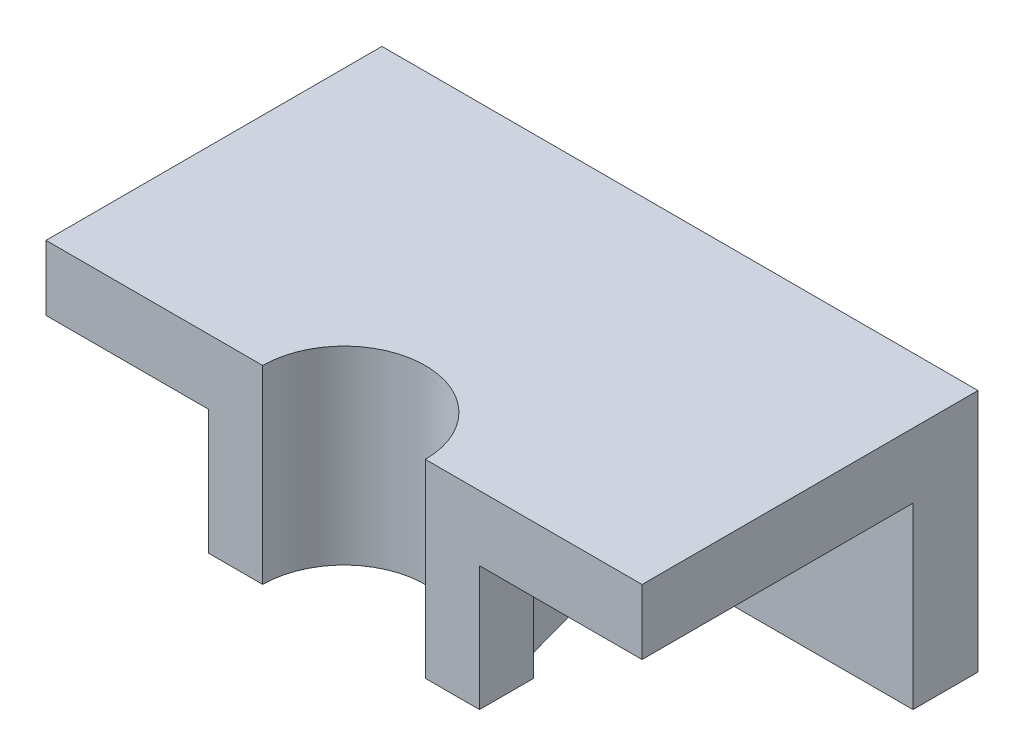
ISO-10303-21;
HEADER;
FILE_DESCRIPTION(('STEP AP214'),'2;1');
FILE_NAME('part.step','',(''),(''),'','','');
FILE_SCHEMA(('AUTOMOTIVE_DESIGN { 1 0 10303 214 1 1 1 1 }'));
ENDSEC;
DATA;
#1=APPLICATION_CONTEXT('core data for automotive mechanical design processes');
#2=APPLICATION_PROTOCOL_DEFINITION('international standard','automotive_design',2000,#1);
#3=PRODUCT_CONTEXT('',#1,'mechanical');
#4=PRODUCT('Part','Part','',(#3));
#5=PRODUCT_RELATED_PRODUCT_CATEGORY('part','',(#4));
#6=PRODUCT_DEFINITION_FORMATION('','',#4);
#7=PRODUCT_DEFINITION_CONTEXT('part definition',#1,'design');
#8=PRODUCT_DEFINITION('design','',#6,#7);
#9=PRODUCT_DEFINITION_SHAPE('','',#8);
#10=(LENGTH_UNIT() NAMED_UNIT(*) SI_UNIT(.MILLI.,.METRE.));
#11=(NAMED_UNIT(*) PLANE_ANGLE_UNIT() SI_UNIT($,.RADIAN.));
#12=(NAMED_UNIT(*) SI_UNIT($,.STERADIAN.) SOLID_ANGLE_UNIT());
#13=UNCERTAINTY_MEASURE_WITH_UNIT(LENGTH_MEASURE(1.E-05),#10,'distance_accuracy_value','');
#14=(GEOMETRIC_REPRESENTATION_CONTEXT(3) GLOBAL_UNCERTAINTY_ASSIGNED_CONTEXT((#13)) GLOBAL_UNIT_ASSIGNED_CONTEXT((#10,
#11,#12)) REPRESENTATION_CONTEXT('',''));
#15=CARTESIAN_POINT('',(0.,0.,0.));
#16=DIRECTION('',(0.,0.,1.));
#17=DIRECTION('',(1.,0.,0.));
#18=AXIS2_PLACEMENT_3D('',#15,#16,#17);
#19=CARTESIAN_POINT('',(110.,33.,62.));
#20=DIRECTION('',(0.,0.,1.));
#21=DIRECTION('',(1.,0.,0.));
#22=AXIS2_PLACEMENT_3D('',#19,#20,#21);
#23=PLANE('',#22);
#24=DIRECTION('',(0.,1.,0.));
#25=VECTOR('',#24,1.);
#26=CARTESIAN_POINT('',(40.,10.,62.));
#27=LINE('',#26,#25);
#28=CARTESIAN_POINT('',(40.,10.,62.));
#29=VERTEX_POINT('',#28);
#30=CARTESIAN_POINT('',(40.,45.,61.9999999999999));
#31=VERTEX_POINT('',#30);
#32=EDGE_CURVE('E179',#29,#31,#27,.T.);
#33=ORIENTED_EDGE('',*,*,#32,.T.);
#34=DIRECTION('',(1.,0.,0.));
#35=VECTOR('',#34,1.);
#36=CARTESIAN_POINT('',(110.,45.,62.));
#37=LINE('',#36,#35);
#38=CARTESIAN_POINT('',(0.,45.,62.));
#39=VERTEX_POINT('',#38);
#40=EDGE_CURVE('E140',#39,#31,#37,.T.);
#41=ORIENTED_EDGE('',*,*,#40,.F.);
#42=DIRECTION('',(0.,1.,0.));
#43=VECTOR('',#42,1.);
#44=CARTESIAN_POINT('',(0.,33.,62.));
#45=LINE('',#44,#43);
#46=CARTESIAN_POINT('',(0.,33.,62.));
#47=VERTEX_POINT('',#46);
#48=EDGE_CURVE('E108',#47,#39,#45,.T.);
#49=ORIENTED_EDGE('',*,*,#48,.F.);
#50=DIRECTION('',(1.,0.,0.));
#51=VECTOR('',#50,1.);
#52=CARTESIAN_POINT('',(110.,33.,62.));
#53=LINE('',#52,#51);
#54=CARTESIAN_POINT('',(30.,33.,62.));
#55=VERTEX_POINT('',#54);
#56=EDGE_CURVE('E142',#47,#55,#53,.T.);
#57=ORIENTED_EDGE('',*,*,#56,.T.);
#58=DIRECTION('',(0.,1.,0.));
#59=VECTOR('',#58,1.);
#60=CARTESIAN_POINT('',(30.,10.,62.));
#61=LINE('',#60,#59);
#62=CARTESIAN_POINT('',(30.,10.,62.));
#63=VERTEX_POINT('',#62);
#64=EDGE_CURVE('E147',#63,#55,#61,.T.);
#65=ORIENTED_EDGE('',*,*,#64,.F.);
#66=DIRECTION('',(-1.,0.,0.));
#67=VECTOR('',#66,1.);
#68=CARTESIAN_POINT('',(30.,10.,62.));
#69=LINE('',#68,#67);
#70=EDGE_CURVE('E181',#29,#63,#69,.T.);
#71=ORIENTED_EDGE('',*,*,#70,.F.);
#72=EDGE_LOOP('',(#33,#41,#49,#57,#65,#71));
#73=FACE_BOUND('',#72,.T.);
#74=ADVANCED_FACE('F44',(#73),#23,.T.);
#75=CARTESIAN_POINT('',(0.,0.,12.));
#76=DIRECTION('',(0.,0.,1.));
#77=DIRECTION('',(1.,0.,0.));
#78=AXIS2_PLACEMENT_3D('',#75,#76,#77);
#79=PLANE('',#78);
#80=DIRECTION('',(1.,0.,0.));
#81=VECTOR('',#80,1.);
#82=CARTESIAN_POINT('',(55.,10.,12.));
#83=LINE('',#82,#81);
#84=CARTESIAN_POINT('',(44.,10.,12.));
#85=VERTEX_POINT('',#84);
#86=CARTESIAN_POINT('',(66.,10.,12.));
#87=VERTEX_POINT('',#86);
#88=EDGE_CURVE('E212',#85,#87,#83,.T.);
#89=ORIENTED_EDGE('',*,*,#88,.F.);
#90=DIRECTION('',(0.,1.,0.));
#91=VECTOR('',#90,1.);
#92=CARTESIAN_POINT('',(44.,10.,12.));
#93=LINE('',#92,#91);
#94=CARTESIAN_POINT('',(44.,33.,12.));
#95=VERTEX_POINT('',#94);
#96=EDGE_CURVE('E157',#85,#95,#93,.T.);
#97=ORIENTED_EDGE('',*,*,#96,.T.);
#98=DIRECTION('',(-1.,0.,0.));
#99=VECTOR('',#98,1.);
#100=CARTESIAN_POINT('',(0.,33.,12.));
#101=LINE('',#100,#99);
#102=CARTESIAN_POINT('',(0.,33.,12.));
#103=VERTEX_POINT('',#102);
#104=EDGE_CURVE('E58',#95,#103,#101,.T.);
#105=ORIENTED_EDGE('',*,*,#104,.T.);
#106=DIRECTION('',(0.,-1.,0.));
#107=VECTOR('',#106,1.);
#108=CARTESIAN_POINT('',(0.,45.,12.));
#109=LINE('',#108,#107);
#110=CARTESIAN_POINT('',(0.,0.,12.));
#111=VERTEX_POINT('',#110);
#112=EDGE_CURVE('E99',#103,#111,#109,.T.);
#113=ORIENTED_EDGE('',*,*,#112,.T.);
#114=DIRECTION('',(1.,0.,0.));
#115=VECTOR('',#114,1.);
#116=CARTESIAN_POINT('',(0.,0.,12.));
#117=LINE('',#116,#115);
#118=CARTESIAN_POINT('',(110.,0.,12.));
#119=VERTEX_POINT('',#118);
#120=EDGE_CURVE('E66',#111,#119,#117,.T.);
#121=ORIENTED_EDGE('',*,*,#120,.T.);
#122=DIRECTION('',(0.,1.,0.));
#123=VECTOR('',#122,1.);
#124=CARTESIAN_POINT('',(110.,0.,12.));
#125=LINE('',#124,#123);
#126=CARTESIAN_POINT('',(110.,33.,12.));
#127=VERTEX_POINT('',#126);
#128=EDGE_CURVE('E112',#119,#127,#125,.T.);
#129=ORIENTED_EDGE('',*,*,#128,.T.);
#130=CARTESIAN_POINT('',(66.,33.,12.));
#131=VERTEX_POINT('',#130);
#132=EDGE_CURVE('E150',#127,#131,#101,.T.);
#133=ORIENTED_EDGE('',*,*,#132,.T.);
#134=DIRECTION('',(0.,1.,0.));
#135=VECTOR('',#134,1.);
#136=CARTESIAN_POINT('',(66.,10.,12.));
#137=LINE('',#136,#135);
#138=EDGE_CURVE('E161',#87,#131,#137,.T.);
#139=ORIENTED_EDGE('',*,*,#138,.F.);
#140=EDGE_LOOP('',(#89,#97,#105,#113,#121,#129,#133,#139));
#141=FACE_BOUND('',#140,.T.);
#142=ADVANCED_FACE('F257',(#141),#79,.T.);
#143=CARTESIAN_POINT('',(0.,33.,0.));
#144=DIRECTION('',(0.,-1.,0.));
#145=DIRECTION('',(0.,0.,-1.));
#146=AXIS2_PLACEMENT_3D('',#143,#144,#145);
#147=PLANE('',#146);
#148=DIRECTION('',(1.,0.,0.));
#149=VECTOR('',#148,1.);
#150=CARTESIAN_POINT('',(30.,33.,52.));
#151=LINE('',#150,#149);
#152=CARTESIAN_POINT('',(30.,33.,52.));
#153=VERTEX_POINT('',#152);
#154=CARTESIAN_POINT('',(33.,33.,52.));
#155=VERTEX_POINT('',#154);
#156=EDGE_CURVE('E195',#153,#155,#151,.T.);
#157=ORIENTED_EDGE('',*,*,#156,.F.);
#158=DIRECTION('',(0.,0.,-1.));
#159=VECTOR('',#158,1.);
#160=CARTESIAN_POINT('',(30.,33.,52.));
#161=LINE('',#160,#159);
#162=EDGE_CURVE('E198',#55,#153,#161,.T.);
#163=ORIENTED_EDGE('',*,*,#162,.F.);
#164=ORIENTED_EDGE('',*,*,#56,.F.);
#165=DIRECTION('',(0.,0.,1.));
#166=VECTOR('',#165,1.);
#167=CARTESIAN_POINT('',(0.,33.,62.));
#168=LINE('',#167,#166);
#169=EDGE_CURVE('E134',#103,#47,#168,.T.);
#170=ORIENTED_EDGE('',*,*,#169,.F.);
#171=ORIENTED_EDGE('',*,*,#104,.F.);
#172=DIRECTION('',(0.265156483021042,0.,-0.96420539280379));
#173=VECTOR('',#172,1.);
#174=CARTESIAN_POINT('',(33.,33.,52.));
#175=LINE('',#174,#173);
#176=EDGE_CURVE('E190',#155,#95,#175,.T.);
#177=ORIENTED_EDGE('',*,*,#176,.F.);
#178=EDGE_LOOP('',(#157,#163,#164,#170,#171,#177));
#179=FACE_BOUND('',#178,.T.);
#180=ADVANCED_FACE('F304',(#179),#147,.T.);
#181=DIRECTION('',(1.,0.,0.));
#182=VECTOR('',#181,1.);
#183=CARTESIAN_POINT('',(77.,33.,52.));
#184=LINE('',#183,#182);
#185=CARTESIAN_POINT('',(77.,33.,52.));
#186=VERTEX_POINT('',#185);
#187=CARTESIAN_POINT('',(80.,33.,52.));
#188=VERTEX_POINT('',#187);
#189=EDGE_CURVE('E184',#186,#188,#184,.T.);
#190=ORIENTED_EDGE('',*,*,#189,.F.);
#191=DIRECTION('',(0.265156483021042,0.,0.96420539280379));
#192=VECTOR('',#191,1.);
#193=CARTESIAN_POINT('',(66.,33.,12.));
#194=LINE('',#193,#192);
#195=EDGE_CURVE('E187',#131,#186,#194,.T.);
#196=ORIENTED_EDGE('',*,*,#195,.F.);
#197=ORIENTED_EDGE('',*,*,#132,.F.);
#198=DIRECTION('',(0.,0.,-1.));
#199=VECTOR('',#198,1.);
#200=CARTESIAN_POINT('',(110.,33.,12.));
#201=LINE('',#200,#199);
#202=CARTESIAN_POINT('',(110.,33.,62.));
#203=VERTEX_POINT('',#202);
#204=EDGE_CURVE('E139',#203,#127,#201,.T.);
#205=ORIENTED_EDGE('',*,*,#204,.F.);
#206=CARTESIAN_POINT('',(80.,33.,62.));
#207=VERTEX_POINT('',#206);
#208=EDGE_CURVE('E144',#207,#203,#53,.T.);
#209=ORIENTED_EDGE('',*,*,#208,.F.);
#210=DIRECTION('',(0.,0.,1.));
#211=VECTOR('',#210,1.);
#212=CARTESIAN_POINT('',(80.,33.,62.));
#213=LINE('',#212,#211);
#214=EDGE_CURVE('E177',#188,#207,#213,.T.);
#215=ORIENTED_EDGE('',*,*,#214,.F.);
#216=EDGE_LOOP('',(#190,#196,#197,#205,#209,#215));
#217=FACE_BOUND('',#216,.T.);
#218=ADVANCED_FACE('F252',(#217),#147,.T.);
#219=CARTESIAN_POINT('',(0.,45.,12.));
#220=DIRECTION('',(1.,0.,0.));
#221=DIRECTION('',(0.,0.,-1.));
#222=AXIS2_PLACEMENT_3D('',#219,#220,#221);
#223=PLANE('',#222);
#224=DIRECTION('',(0.,-1.,0.));
#225=VECTOR('',#224,1.);
#226=CARTESIAN_POINT('',(0.,45.,0.));
#227=LINE('',#226,#225);
#228=CARTESIAN_POINT('',(0.,45.,0.));
#229=VERTEX_POINT('',#228);
#230=CARTESIAN_POINT('',(0.,0.,0.));
#231=VERTEX_POINT('',#230);
#232=EDGE_CURVE('E106',#229,#231,#227,.T.);
#233=ORIENTED_EDGE('',*,*,#232,.T.);
#234=DIRECTION('',(0.,0.,-1.));
#235=VECTOR('',#234,1.);
#236=CARTESIAN_POINT('',(0.,0.,12.));
#237=LINE('',#236,#235);
#238=EDGE_CURVE('E11',#111,#231,#237,.T.);
#239=ORIENTED_EDGE('',*,*,#238,.F.);
#240=ORIENTED_EDGE('',*,*,#112,.F.);
#241=ORIENTED_EDGE('',*,*,#169,.T.);
#242=ORIENTED_EDGE('',*,*,#48,.T.);
#243=DIRECTION('',(0.,0.,-1.));
#244=VECTOR('',#243,1.);
#245=CARTESIAN_POINT('',(0.,45.,12.));
#246=LINE('',#245,#244);
#247=EDGE_CURVE('E95',#39,#229,#246,.T.);
#248=ORIENTED_EDGE('',*,*,#247,.T.);
#249=EDGE_LOOP('',(#233,#239,#240,#241,#242,#248));
#250=FACE_BOUND('',#249,.T.);
#251=ADVANCED_FACE('F50',(#250),#223,.F.);
#252=CARTESIAN_POINT('',(0.,0.,12.));
#253=DIRECTION('',(0.,1.,0.));
#254=DIRECTION('',(0.,0.,1.));
#255=AXIS2_PLACEMENT_3D('',#252,#253,#254);
#256=PLANE('',#255);
#257=DIRECTION('',(1.,0.,0.));
#258=VECTOR('',#257,1.);
#259=CARTESIAN_POINT('',(0.,0.,0.));
#260=LINE('',#259,#258);
#261=CARTESIAN_POINT('',(110.,0.,0.));
#262=VERTEX_POINT('',#261);
#263=EDGE_CURVE('E111',#231,#262,#260,.T.);
#264=ORIENTED_EDGE('',*,*,#263,.T.);
#265=DIRECTION('',(0.,0.,-1.));
#266=VECTOR('',#265,1.);
#267=CARTESIAN_POINT('',(110.,0.,12.));
#268=LINE('',#267,#266);
#269=EDGE_CURVE('E52',#119,#262,#268,.T.);
#270=ORIENTED_EDGE('',*,*,#269,.F.);
#271=ORIENTED_EDGE('',*,*,#120,.F.);
#272=ORIENTED_EDGE('',*,*,#238,.T.);
#273=EDGE_LOOP('',(#264,#270,#271,#272));
#274=FACE_BOUND('',#273,.T.);
#275=ADVANCED_FACE('F128',(#274),#256,.F.);
#276=CARTESIAN_POINT('',(110.,0.,12.));
#277=DIRECTION('',(-1.,0.,0.));
#278=DIRECTION('',(0.,0.,1.));
#279=AXIS2_PLACEMENT_3D('',#276,#277,#278);
#280=PLANE('',#279);
#281=DIRECTION('',(0.,1.,0.));
#282=VECTOR('',#281,1.);
#283=CARTESIAN_POINT('',(110.,0.,0.));
#284=LINE('',#283,#282);
#285=CARTESIAN_POINT('',(110.,45.,0.));
#286=VERTEX_POINT('',#285);
#287=EDGE_CURVE('E101',#262,#286,#284,.T.);
#288=ORIENTED_EDGE('',*,*,#287,.T.);
#289=DIRECTION('',(0.,0.,-1.));
#290=VECTOR('',#289,1.);
#291=CARTESIAN_POINT('',(110.,45.,12.));
#292=LINE('',#291,#290);
#293=CARTESIAN_POINT('',(110.,45.,62.));
#294=VERTEX_POINT('',#293);
#295=EDGE_CURVE('E96',#294,#286,#292,.T.);
#296=ORIENTED_EDGE('',*,*,#295,.F.);
#297=DIRECTION('',(0.,1.,0.));
#298=VECTOR('',#297,1.);
#299=CARTESIAN_POINT('',(110.,33.,62.));
#300=LINE('',#299,#298);
#301=EDGE_CURVE('E113',#203,#294,#300,.T.);
#302=ORIENTED_EDGE('',*,*,#301,.F.);
#303=ORIENTED_EDGE('',*,*,#204,.T.);
#304=ORIENTED_EDGE('',*,*,#128,.F.);
#305=ORIENTED_EDGE('',*,*,#269,.T.);
#306=EDGE_LOOP('',(#288,#296,#302,#303,#304,#305));
#307=FACE_BOUND('',#306,.T.);
#308=ADVANCED_FACE('F130',(#307),#280,.F.);
#309=CARTESIAN_POINT('',(110.,45.,12.));
#310=DIRECTION('',(0.,-1.,0.));
#311=DIRECTION('',(0.,0.,-1.));
#312=AXIS2_PLACEMENT_3D('',#309,#310,#311);
#313=PLANE('',#312);
#314=ORIENTED_EDGE('',*,*,#40,.T.);
#315=CARTESIAN_POINT('',(55.,45.,62.));
#316=DIRECTION('',(0.,-1.,0.));
#317=DIRECTION('',(0.,0.,-1.));
#318=AXIS2_PLACEMENT_3D('',#315,#316,#317);
#319=CIRCLE('',#318,15.);
#320=CARTESIAN_POINT('',(70.,45.,62.));
#321=VERTEX_POINT('',#320);
#322=EDGE_CURVE('E200',#31,#321,#319,.T.);
#323=ORIENTED_EDGE('',*,*,#322,.T.);
#324=EDGE_CURVE('E137',#321,#294,#37,.T.);
#325=ORIENTED_EDGE('',*,*,#324,.T.);
#326=ORIENTED_EDGE('',*,*,#295,.T.);
#327=DIRECTION('',(-1.,0.,0.));
#328=VECTOR('',#327,1.);
#329=CARTESIAN_POINT('',(110.,45.,0.));
#330=LINE('',#329,#328);
#331=EDGE_CURVE('E87',#286,#229,#330,.T.);
#332=ORIENTED_EDGE('',*,*,#331,.T.);
#333=ORIENTED_EDGE('',*,*,#247,.F.);
#334=EDGE_LOOP('',(#314,#323,#325,#326,#332,#333));
#335=FACE_BOUND('',#334,.T.);
#336=ADVANCED_FACE('F89',(#335),#313,.F.);
#337=CARTESIAN_POINT('',(0.,0.,0.));
#338=DIRECTION('',(0.,0.,1.));
#339=DIRECTION('',(1.,0.,0.));
#340=AXIS2_PLACEMENT_3D('',#337,#338,#339);
#341=PLANE('',#340);
#342=ORIENTED_EDGE('',*,*,#232,.F.);
#343=ORIENTED_EDGE('',*,*,#331,.F.);
#344=ORIENTED_EDGE('',*,*,#287,.F.);
#345=ORIENTED_EDGE('',*,*,#263,.F.);
#346=EDGE_LOOP('',(#342,#343,#344,#345));
#347=FACE_BOUND('',#346,.T.);
#348=ADVANCED_FACE('F114',(#347),#341,.F.);
#349=ORIENTED_EDGE('',*,*,#324,.F.);
#350=DIRECTION('',(0.,1.,0.));
#351=VECTOR('',#350,1.);
#352=CARTESIAN_POINT('',(70.,10.,62.));
#353=LINE('',#352,#351);
#354=CARTESIAN_POINT('',(70.,10.,62.));
#355=VERTEX_POINT('',#354);
#356=EDGE_CURVE('E174',#355,#321,#353,.T.);
#357=ORIENTED_EDGE('',*,*,#356,.F.);
#358=DIRECTION('',(-1.,0.,0.));
#359=VECTOR('',#358,1.);
#360=CARTESIAN_POINT('',(70.,10.,62.));
#361=LINE('',#360,#359);
#362=CARTESIAN_POINT('',(80.,10.,62.));
#363=VERTEX_POINT('',#362);
#364=EDGE_CURVE('E205',#363,#355,#361,.T.);
#365=ORIENTED_EDGE('',*,*,#364,.F.);
#366=DIRECTION('',(0.,1.,0.));
#367=VECTOR('',#366,1.);
#368=CARTESIAN_POINT('',(80.,10.,62.));
#369=LINE('',#368,#367);
#370=EDGE_CURVE('E168',#363,#207,#369,.T.);
#371=ORIENTED_EDGE('',*,*,#370,.T.);
#372=ORIENTED_EDGE('',*,*,#208,.T.);
#373=ORIENTED_EDGE('',*,*,#301,.T.);
#374=EDGE_LOOP('',(#349,#357,#365,#371,#372,#373));
#375=FACE_BOUND('',#374,.T.);
#376=ADVANCED_FACE('F239',(#375),#23,.T.);
#377=CARTESIAN_POINT('',(30.,10.,52.));
#378=DIRECTION('',(1.,0.,0.));
#379=DIRECTION('',(0.,0.,-1.));
#380=AXIS2_PLACEMENT_3D('',#377,#378,#379);
#381=PLANE('',#380);
#382=ORIENTED_EDGE('',*,*,#162,.T.);
#383=DIRECTION('',(0.,1.,0.));
#384=VECTOR('',#383,1.);
#385=CARTESIAN_POINT('',(30.,10.,52.));
#386=LINE('',#385,#384);
#387=CARTESIAN_POINT('',(30.,10.,52.));
#388=VERTEX_POINT('',#387);
#389=EDGE_CURVE('E153',#388,#153,#386,.T.);
#390=ORIENTED_EDGE('',*,*,#389,.F.);
#391=DIRECTION('',(0.,0.,-1.));
#392=VECTOR('',#391,1.);
#393=CARTESIAN_POINT('',(30.,10.,52.));
#394=LINE('',#393,#392);
#395=EDGE_CURVE('E224',#63,#388,#394,.T.);
#396=ORIENTED_EDGE('',*,*,#395,.F.);
#397=ORIENTED_EDGE('',*,*,#64,.T.);
#398=EDGE_LOOP('',(#382,#390,#396,#397));
#399=FACE_BOUND('',#398,.T.);
#400=ADVANCED_FACE('F328',(#399),#381,.F.);
#401=CARTESIAN_POINT('',(30.,10.,52.));
#402=DIRECTION('',(0.,0.,1.));
#403=DIRECTION('',(1.,0.,0.));
#404=AXIS2_PLACEMENT_3D('',#401,#402,#403);
#405=PLANE('',#404);
#406=ORIENTED_EDGE('',*,*,#156,.T.);
#407=DIRECTION('',(0.,1.,0.));
#408=VECTOR('',#407,1.);
#409=CARTESIAN_POINT('',(33.,10.,52.));
#410=LINE('',#409,#408);
#411=CARTESIAN_POINT('',(33.,10.,52.));
#412=VERTEX_POINT('',#411);
#413=EDGE_CURVE('E156',#412,#155,#410,.T.);
#414=ORIENTED_EDGE('',*,*,#413,.F.);
#415=DIRECTION('',(1.,0.,0.));
#416=VECTOR('',#415,1.);
#417=CARTESIAN_POINT('',(30.,10.,52.));
#418=LINE('',#417,#416);
#419=EDGE_CURVE('E219',#388,#412,#418,.T.);
#420=ORIENTED_EDGE('',*,*,#419,.F.);
#421=ORIENTED_EDGE('',*,*,#389,.T.);
#422=EDGE_LOOP('',(#406,#414,#420,#421));
#423=FACE_BOUND('',#422,.T.);
#424=ADVANCED_FACE('F287',(#423),#405,.F.);
#425=CARTESIAN_POINT('',(33.,10.,52.));
#426=DIRECTION('',(0.96420539280379,0.,0.265156483021042));
#427=DIRECTION('',(0.265156483021042,0.,-0.96420539280379));
#428=AXIS2_PLACEMENT_3D('',#425,#426,#427);
#429=PLANE('',#428);
#430=ORIENTED_EDGE('',*,*,#176,.T.);
#431=ORIENTED_EDGE('',*,*,#96,.F.);
#432=DIRECTION('',(0.265156483021042,0.,-0.96420539280379));
#433=VECTOR('',#432,1.);
#434=CARTESIAN_POINT('',(33.,10.,52.));
#435=LINE('',#434,#433);
#436=EDGE_CURVE('E220',#412,#85,#435,.T.);
#437=ORIENTED_EDGE('',*,*,#436,.F.);
#438=ORIENTED_EDGE('',*,*,#413,.T.);
#439=EDGE_LOOP('',(#430,#431,#437,#438));
#440=FACE_BOUND('',#439,.T.);
#441=ADVANCED_FACE('F298',(#440),#429,.F.);
#442=CARTESIAN_POINT('',(66.,10.,12.));
#443=DIRECTION('',(-0.96420539280379,0.,0.265156483021042));
#444=DIRECTION('',(0.265156483021042,0.,0.96420539280379));
#445=AXIS2_PLACEMENT_3D('',#442,#443,#444);
#446=PLANE('',#445);
#447=ORIENTED_EDGE('',*,*,#195,.T.);
#448=DIRECTION('',(0.,1.,0.));
#449=VECTOR('',#448,1.);
#450=CARTESIAN_POINT('',(77.,10.,52.));
#451=LINE('',#450,#449);
#452=CARTESIAN_POINT('',(77.,10.,52.));
#453=VERTEX_POINT('',#452);
#454=EDGE_CURVE('E163',#453,#186,#451,.T.);
#455=ORIENTED_EDGE('',*,*,#454,.F.);
#456=DIRECTION('',(0.265156483021042,0.,0.96420539280379));
#457=VECTOR('',#456,1.);
#458=CARTESIAN_POINT('',(66.,10.,12.));
#459=LINE('',#458,#457);
#460=EDGE_CURVE('E211',#87,#453,#459,.T.);
#461=ORIENTED_EDGE('',*,*,#460,.F.);
#462=ORIENTED_EDGE('',*,*,#138,.T.);
#463=EDGE_LOOP('',(#447,#455,#461,#462));
#464=FACE_BOUND('',#463,.T.);
#465=ADVANCED_FACE('F358',(#464),#446,.F.);
#466=CARTESIAN_POINT('',(77.,10.,52.));
#467=DIRECTION('',(0.,0.,1.));
#468=DIRECTION('',(1.,0.,0.));
#469=AXIS2_PLACEMENT_3D('',#466,#467,#468);
#470=PLANE('',#469);
#471=ORIENTED_EDGE('',*,*,#189,.T.);
#472=DIRECTION('',(0.,1.,0.));
#473=VECTOR('',#472,1.);
#474=CARTESIAN_POINT('',(80.,10.,52.));
#475=LINE('',#474,#473);
#476=CARTESIAN_POINT('',(80.,10.,52.));
#477=VERTEX_POINT('',#476);
#478=EDGE_CURVE('E170',#477,#188,#475,.T.);
#479=ORIENTED_EDGE('',*,*,#478,.F.);
#480=DIRECTION('',(1.,0.,0.));
#481=VECTOR('',#480,1.);
#482=CARTESIAN_POINT('',(77.,10.,52.));
#483=LINE('',#482,#481);
#484=EDGE_CURVE('E208',#453,#477,#483,.T.);
#485=ORIENTED_EDGE('',*,*,#484,.F.);
#486=ORIENTED_EDGE('',*,*,#454,.T.);
#487=EDGE_LOOP('',(#471,#479,#485,#486));
#488=FACE_BOUND('',#487,.T.);
#489=ADVANCED_FACE('F320',(#488),#470,.F.);
#490=CARTESIAN_POINT('',(80.,10.,62.));
#491=DIRECTION('',(-1.,0.,0.));
#492=DIRECTION('',(0.,0.,1.));
#493=AXIS2_PLACEMENT_3D('',#490,#491,#492);
#494=PLANE('',#493);
#495=ORIENTED_EDGE('',*,*,#214,.T.);
#496=ORIENTED_EDGE('',*,*,#370,.F.);
#497=DIRECTION('',(0.,0.,1.));
#498=VECTOR('',#497,1.);
#499=CARTESIAN_POINT('',(80.,10.,62.));
#500=LINE('',#499,#498);
#501=EDGE_CURVE('E202',#477,#363,#500,.T.);
#502=ORIENTED_EDGE('',*,*,#501,.F.);
#503=ORIENTED_EDGE('',*,*,#478,.T.);
#504=EDGE_LOOP('',(#495,#496,#502,#503));
#505=FACE_BOUND('',#504,.T.);
#506=ADVANCED_FACE('F309',(#505),#494,.F.);
#507=CARTESIAN_POINT('',(55.,10.,62.));
#508=DIRECTION('',(0.,1.,0.));
#509=DIRECTION('',(0.,0.,1.));
#510=AXIS2_PLACEMENT_3D('',#507,#508,#509);
#511=CYLINDRICAL_SURFACE('',#510,15.);
#512=ORIENTED_EDGE('',*,*,#356,.T.);
#513=ORIENTED_EDGE('',*,*,#322,.F.);
#514=ORIENTED_EDGE('',*,*,#32,.F.);
#515=CARTESIAN_POINT('',(55.,10.,62.));
#516=DIRECTION('',(0.,1.,0.));
#517=DIRECTION('',(0.,0.,-1.));
#518=AXIS2_PLACEMENT_3D('',#515,#516,#517);
#519=CIRCLE('',#518,15.);
#520=EDGE_CURVE('E178',#355,#29,#519,.T.);
#521=ORIENTED_EDGE('',*,*,#520,.F.);
#522=EDGE_LOOP('',(#512,#513,#514,#521));
#523=FACE_BOUND('',#522,.T.);
#524=ADVANCED_FACE('F307',(#523),#511,.F.);
#525=CARTESIAN_POINT('',(55.,10.,62.));
#526=DIRECTION('',(0.,-1.,0.));
#527=DIRECTION('',(0.,0.,-1.));
#528=AXIS2_PLACEMENT_3D('',#525,#526,#527);
#529=PLANE('',#528);
#530=ORIENTED_EDGE('',*,*,#70,.T.);
#531=ORIENTED_EDGE('',*,*,#395,.T.);
#532=ORIENTED_EDGE('',*,*,#419,.T.);
#533=ORIENTED_EDGE('',*,*,#436,.T.);
#534=ORIENTED_EDGE('',*,*,#88,.T.);
#535=ORIENTED_EDGE('',*,*,#460,.T.);
#536=ORIENTED_EDGE('',*,*,#484,.T.);
#537=ORIENTED_EDGE('',*,*,#501,.T.);
#538=ORIENTED_EDGE('',*,*,#364,.T.);
#539=ORIENTED_EDGE('',*,*,#520,.T.);
#540=EDGE_LOOP('',(#530,#531,#532,#533,#534,#535,#536,#537,#538,#539));
#541=FACE_BOUND('',#540,.T.);
#542=ADVANCED_FACE('F310',(#541),#529,.T.);
#543=CLOSED_SHELL('',(#74,#142,#180,#218,#251,#275,#308,#336,#348,#376,#400,#424,#441,#465,#489,
#506,#524,#542));
#544=MANIFOLD_SOLID_BREP('B2',#543);
#545=ADVANCED_BREP_SHAPE_REPRESENTATION('',(#18,#544),#14);
#546=SHAPE_DEFINITION_REPRESENTATION(#9,#545);
ENDSEC;
END-ISO-10303-21;
